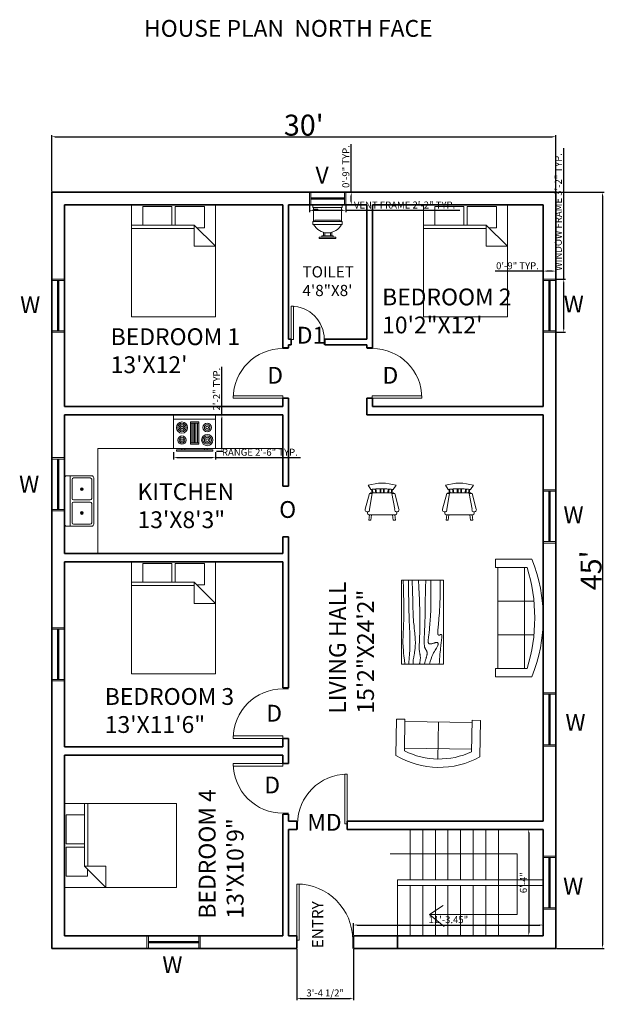
# Model space of a CAD drawing. Units: inches. Extents: x 1662 to 23131, y 1265 to 19127.
# Tile 1 of 26: x 2071 to 2489, y 1265 to 1968. Entities that reach past the tile are written whole.
import ezdxf

# ---------------------------------------------------------------- set-up
doc = ezdxf.new("R2010")
doc.units = ezdxf.units.IN
for name, color, linetype, lineweight in [('A-ANNO-DIMS', 4, 'Continuous', 18), ('A-ANNO-IDEN', 7, 'Continuous', 18), ('A-ANNO-TITL', 7, 'Continuous', 35), ('A-AREA-IDEN', 7, 'Continuous', 18), ('A-DOOR', 3, 'Continuous', 18), ('A-EQPM', 8, 'Continuous', 18), ('A-FLOR-CASE', 8, 'Continuous', 18), ('A-FLOR-FIXT', 9, 'Continuous', 18), ('A-FLOR-STRS', 7, 'Continuous', 18), ('A-FURN', 8, 'Continuous', 18), ('A-GLAZ', 4, 'Continuous', 18), ('A-WALL', 7, 'Continuous', 35)]:
    doc.layers.add(name, color=color, linetype=linetype, lineweight=lineweight)
doc.styles.get("Standard").update_dxf_attribs({"font": 'arial.ttf'})
doc.dimstyles.new('ISO-25', dxfattribs={"dimtxt": 5, "dimasz": 2.5, "dimexe": 1.25, "dimexo": 0.625, "dimtad": 1, "dimlunit": 3, "dimtxsty": 'Standard', "dimcen": 2.5, "dimadec": 0, "dimazin": 0, "dimtfac": 1, "dimtmove": 0, "dimatfit": 3, "dimfxl": 1, "dimarcsym": 0})

# ---------------------------------------------------------------- blocks, each defined once
blk = doc.blocks.new('*D1')
at = {"layer": 'A-ANNO-DIMS', "color": 0, "lineweight": -2, "transparency": 16777216}
for p, q in [((2094.29, 1845.35), (2094.29, 1885.6)), ((2454.29, 1845.35), (2454.29, 1885.6)), ((2096.79, 1884.35), (2451.79, 1884.35))]:
    blk.add_line(p, q, dxfattribs=at)
at = {"layer": 'A-ANNO-DIMS', "color": 0, "transparency": 16777216}
for points in [[(2096.79, 1884.76), (2096.79, 1883.93), (2094.29, 1884.35)], [(2451.79, 1884.76), (2451.79, 1883.93), (2454.29, 1884.35)]]:
    blk.add_solid(points, dxfattribs=at)
at = {"layer": 'Defpoints', "color": 0, "transparency": 16777216}
for p in [(2454.29, 1884.35), (2094.29, 1844.72), (2454.29, 1844.72)]:
    blk.add_point(p, dxfattribs=at)
at = {"layer": 'A-ANNO-DIMS', "color": 0, "transparency": 16777216, "insert": (2274.29, 1892.63), "char_height": 5, "attachment_point": 5}
blk.add_mtext("{\\H3x;30'}", dxfattribs=at)
blk = doc.blocks.new('*D2')
at = {"layer": 'A-ANNO-DIMS', "color": 0, "lineweight": -2, "transparency": 16777216}
for p, q in [((2454.92, 1844.72), (2488.97, 1844.72)), ((2487.72, 1842.22), (2487.72, 1307.22)), ((2454.92, 1304.72), (2488.97, 1304.72))]:
    blk.add_line(p, q, dxfattribs=at)
at = {"layer": 'A-ANNO-DIMS', "color": 0, "transparency": 16777216}
for points in [[(2487.3, 1842.22), (2488.13, 1842.22), (2487.72, 1844.72)], [(2487.3, 1307.22), (2488.13, 1307.22), (2487.72, 1304.72)]]:
    blk.add_solid(points, dxfattribs=at)
at = {"layer": 'Defpoints', "color": 0, "transparency": 16777216}
for p in [(2454.29, 1844.72), (2454.29, 1304.72), (2487.72, 1304.72)]:
    blk.add_point(p, dxfattribs=at)
at = {"layer": 'A-ANNO-DIMS', "color": 0, "transparency": 16777216, "insert": (2479.46, 1574.72), "char_height": 5, "attachment_point": 5, "rotation": 90}
blk.add_mtext("{\\H3x;45'}", dxfattribs=at)
blk = doc.blocks.new('*U4')
for p, q in [((0, 0), (0, -100)), ((-900, 0), (-900, -100))]:
    blk.add_line(p, q)
blk.add_lwpolyline([(0, 0), (0, 900), (-43.75, 900), (-43.75, 0)], close=True)
blk.add_arc((0, 0), 900, 90, 180)
blk = doc.blocks.new('*U5')
for p, q in [((-900, 0), (-900, 100)), ((0, 0), (0, 100))]:
    blk.add_line(p, q)
blk.add_lwpolyline([(0, 0), (0, -900), (-43.75, -900), (-43.75, 0)], close=True)
blk.add_arc((0, 0), 900, 180, 270)
blk = doc.blocks.new('*U6')
for p, q in [((0, 0), (0, 100)), ((900, 0), (900, 100))]:
    blk.add_line(p, q)
blk.add_lwpolyline([(0, 0), (0, -900), (43.75, -900), (43.75, 0)], close=True)
blk.add_arc((0, 0), 900, 270, 0)
blk = doc.blocks.new('*U7')
for p, q in [((0, 0), (0, -100)), ((-900, 0), (-900, -100))]:
    blk.add_line(p, q)
blk.add_lwpolyline([(0, 0), (0, 900), (-43.75, 900), (-43.75, 0)], close=True)
blk.add_arc((0, 0), 900, 90, 180)
blk = doc.blocks.new('*U8')
for p, q in [((0, 0), (0, -100)), ((600, 0), (600, -100))]:
    blk.add_line(p, q)
blk.add_lwpolyline([(0, 0), (0, 600), (43.75, 600), (43.75, 0)], close=True)
blk.add_arc((0, 0), 600, 0, 90)
blk = doc.blocks.new('*U10')
for p, q in [((0, 0), (0, -6)), ((40, 0), (40, -6))]:
    blk.add_line(p, q)
blk.add_lwpolyline([(0, 0), (0, 40), (1.75, 40), (1.75, 0)], close=True)
blk.add_arc((0, 0), 40, 0, 90)
blk = doc.blocks.new('Chair - Rocking')
for p, q in [((-8, -4.5), (-10, -1.5)), ((-8.23428, -6.99939), (-8.3093, -7.47958)), ((-8.23041, -7), (8.23915, -7)), ((-7.5, -4.5), (-7, -7)), ((-6.5, -7), (-7.02225, -4.43)), ((-4.5, -7), (-4.96674, -4.19951)), ((-4, -7), (-4.40532, -4.16272)), ((-1.5, -4.05012), (-1.5, -7)), ((-1, -7), (-1, -4.05012)), ((1, -7), (1, -4.04655)), ((1.5, -4.05012), (1.5, -7)), ((4, -7), (4.40187, -4.18694)), ((4.5, -7), (4.96761, -4.19437)), ((6.5, -7), (7, -4.4057)), ((7.5, -4.5), (7, -7)), ((8, -4.5), (10, -1.5)), ((8.31071, -7.48854), (8.23449, -7.00073)), ((-9, -7.5), (-12, -18.49999)), ((-7, -7.5), (-9, -7.5)), ((-9, -18.49999), (-7, -7.5)), ((7, -7.5), (9, -7.5)), ((9, -18.49999), (7, -7.5)), ((9, -7.5), (12, -18.49999)), ((-10.36644, -20.64523), (-10.5, -21.49999)), ((10.5, -21.49999), (10.3575, -20.58798)), ((-9, -22.49999), (-9.5, -26.49999)), ((0, -22.49999), (-9.5, -22.49999)), ((-9.5, -26.49999), (-8, -26.49999)), ((-8, -26.49999), (-7.5, -22.49999)), ((0, -22.49999), (9.5, -22.49999)), ((8, -26.49999), (7.5, -22.49999)), ((9.5, -26.49999), (8, -26.49999)), ((9, -22.49999), (9.5, -26.49999))]:
    blk.add_line(p, q)
for centre, radius, start, end in [((0, -34.08333), 34.08333, 72.93847, 107.0615), ((0, -68.25004), 64.25, 93.92211, 97.15267), ((0, -68.25004), 64.25, 82.84733, 93.92211), ((-10.5, -18.99999), 1.58114, 161.5651, 18.43495), ((10.5, -18.99999), 1.58114, 161.5651, 18.43495), ((-9.5, -21.49999), 1, 180, 270), ((9.5, -21.49999), 1, 270, 0)]:
    blk.add_arc(centre, radius, start, end)
blk = doc.blocks.new('Table - Rectangular Woodgrain 60 x 30 in.')
for p, q in [((0, 0), (0, -30)), ((60, 0), (0, 0)), ((60, -30), (60, 0)), ((0, -30), (60, -30))]:
    blk.add_line(p, q)
for points in [[(0, -2.4), (4.8155, -2.418), (9.0302, -2.4688), (12.709, -2.5477), (15.9167, -2.65), (18.7181, -2.7711), (21.1781, -2.9063), (23.3616, -3.0508), (25.3333, -3.2), (27.1477, -3.3495), (28.8172, -3.4958), (30.3437, -3.636), (31.7291, -3.7667), (32.9756, -3.8849), (34.0849, -3.9875), (35.059, -4.0714), (35.9, -4.1334), (36.6114, -4.1711), (37.2041, -4.1854), (37.6906, -4.1779), (38.0833, -4.15), (38.3948, -4.1034), (38.6375, -4.0396), (38.8239, -3.9602), (38.9666, -3.8667), (39.0764, -3.7608), (39.1573, -3.6448), (39.2116, -3.521), (39.2416, -3.3917), (39.2498, -3.2593), (39.2385, -3.1261), (39.21, -2.9944), (39.1666, -2.8667), (39.111, -2.7447), (39.0468, -2.6281), (38.978, -2.5163), (38.9083, -2.4083), (38.8418, -2.3035), (38.7823, -2.201), (38.7337, -2.1001), (38.7, -2), (38.6844, -1.9003), (38.6875, -1.8021), (38.7094, -1.707), (38.75, -1.6167), (38.8094, -1.5326), (38.8875, -1.4563), (38.9844, -1.3893), (39.1, -1.3333), (39.2351, -1.2896), (39.3937, -1.2583), (39.5804, -1.2396), (39.8, -1.2333), (40.057, -1.2396), (40.3562, -1.2583), (40.7023, -1.2896), (41.1, -1.3333), (41.5547, -1.3895), (42.0755, -1.4573), (42.6721, -1.5361), (43.3542, -1.625), (44.1316, -1.7233), (45.014, -1.8302), (46.0114, -1.9449), (47.1333, -2.0667), (48.3862, -2.1947), (49.7625, -2.3281), (51.2513, -2.4663), (52.8416, -2.6083), (54.5226, -2.7535), (56.2833, -2.9011), (58.1127, -3.0501), (60, -3.2)], [(0, -9.2), (6.5759, -9.0858), (11.9385, -9.0365), (16.2527, -9.0418), (19.6833, -9.0917), (22.3952, -9.1759), (24.5531, -9.2844), (26.322, -9.4069), (27.8666, -9.5333), (29.3241, -9.6553), (30.7203, -9.7719), (32.0532, -9.8837), (33.3208, -9.9917), (34.5213, -10.0965), (35.6526, -10.199), (36.7128, -10.2999), (37.7, -10.4), (38.6129, -10.4996), (39.4531, -10.5969), (40.223, -10.6895), (40.925, -10.775), (41.5613, -10.8512), (42.1344, -10.9156), (42.6465, -10.966), (43.1, -11), (43.4976, -11.0158), (43.8437, -11.0136), (44.143, -10.9942), (44.4, -10.9583), (44.6195, -10.9069), (44.8062, -10.8406), (44.9648, -10.7603), (45.1, -10.6667), (45.2155, -10.5598), (45.3114, -10.4365), (45.3871, -10.2929), (45.4416, -10.125), (45.4743, -9.929), (45.4844, -9.7011), (45.4709, -9.4371), (45.4333, -9.1333), (45.3716, -8.7883), (45.2896, -8.4104), (45.1919, -8.0107), (45.0833, -7.6), (44.9685, -7.1893), (44.8521, -6.7896), (44.7388, -6.4117), (44.6333, -6.0667), (44.54, -5.7628), (44.4614, -5.4979), (44.4001, -5.2675), (44.3583, -5.0667), (44.3384, -4.8909), (44.3427, -4.7354), (44.3736, -4.5956), (44.4333, -4.4667), (44.5236, -4.3453), (44.6427, -4.2333), (44.7884, -4.1339), (44.9583, -4.05), (45.1501, -3.9849), (45.3614, -3.9417), (45.59, -3.9234), (45.8333, -3.9333), (46.0915, -3.9749), (46.3734, -4.0531), (46.6906, -4.1736), (47.0542, -4.3417), (47.4756, -4.5629), (47.9661, -4.8427), (48.5372, -5.1866), (49.2, -5.6), (49.9676, -6.0844), (50.8594, -6.625), (51.8965, -7.2031), (53.1, -7.8), (54.491, -8.3969), (56.0906, -8.975), (57.9199, -9.5156), (60, -10)], [(0, -12.8), (5.1847, -12.9322), (9.6213, -13.0323), (13.3963, -13.1059), (16.5958, -13.1583), (19.3063, -13.1952), (21.614, -13.2219), (23.6054, -13.2439), (25.3666, -13.2667), (26.9728, -13.2947), (28.4531, -13.3281), (29.8256, -13.3663), (31.1083, -13.4083), (32.3191, -13.4535), (33.476, -13.501), (34.597, -13.5501), (35.7, -13.6), (36.7984, -13.6497), (37.8875, -13.6979), (38.9578, -13.743), (40, -13.7833), (41.0047, -13.8174), (41.9625, -13.8438), (42.864, -13.8607), (43.7, -13.8667), (44.4631, -13.8604), (45.1552, -13.8417), (45.7801, -13.8104), (46.3416, -13.7667), (46.8439, -13.7104), (47.2906, -13.6417), (47.6858, -13.5604), (48.0333, -13.4667), (48.3375, -13.3608), (48.6042, -13.2448), (48.8396, -13.121), (49.05, -12.9917), (49.2417, -12.8593), (49.4208, -12.7261), (49.5937, -12.5944), (49.7667, -12.4667), (49.9452, -12.3451), (50.1323, -12.2313), (50.3303, -12.1268), (50.5416, -12.0333), (50.7686, -11.9524), (51.0135, -11.8854), (51.2788, -11.8341), (51.5666, -11.8), (51.8785, -11.7843), (52.2116, -11.7865), (52.562, -11.8059), (52.926, -11.8417), (53.2998, -11.8931), (53.6795, -11.9594), (54.0614, -12.0397), (54.4416, -12.1333), (54.8223, -12.2401), (55.2293, -12.3625), (55.6942, -12.5037), (56.2489, -12.6667), (56.9251, -12.8547), (57.7545, -13.0708), (58.7689, -13.3182), (60, -13.6)], [(0, -18), (5.124, -17.7273), (9.6609, -17.5057), (13.6705, -17.3303), (17.2125, -17.1958), (20.3467, -17.0973), (23.1328, -17.0297), (25.6307, -16.9878), (27.9, -16.9667), (29.9928, -16.9617), (31.9302, -16.9703), (33.7254, -16.9907), (35.3917, -17.0208), (36.9423, -17.0588), (38.3906, -17.1026), (39.7499, -17.1503), (41.0333, -17.2), (42.2519, -17.2496), (43.4073, -17.2969), (44.4986, -17.3395), (45.525, -17.375), (46.4858, -17.4012), (47.3802, -17.4156), (48.2074, -17.416), (48.9667, -17.4), (49.6583, -17.3662), (50.2872, -17.3167), (50.8595, -17.2547), (51.3812, -17.1833), (51.8584, -17.1057), (52.2971, -17.025), (52.7034, -16.9443), (53.0833, -16.8667), (53.443, -16.7951), (53.789, -16.7313), (54.128, -16.6768), (54.4666, -16.6334), (54.8115, -16.6024), (55.1693, -16.5854), (55.5465, -16.5841), (55.95, -16.6), (56.3828, -16.6337), (56.8346, -16.6823), (57.2915, -16.7418), (57.7396, -16.8084), (58.165, -16.878), (58.5539, -16.9469), (58.8924, -17.0111), (59.1666, -17.0667), (59.3679, -17.1107), (59.5078, -17.1438), (59.6032, -17.1675), (59.6708, -17.1833), (59.7275, -17.193), (59.7901, -17.1979), (59.8753, -17.1998), (60, -17.2)], [(0, -22.4), (8.0098, -22.2501), (14.4094, -22.1011), (19.4168, -21.9535), (23.25, -21.8083), (26.1269, -21.6663), (28.2656, -21.5281), (29.884, -21.3947), (31.2, -21.2667), (32.3967, -21.1448), (33.5172, -21.0292), (34.5697, -20.9198), (35.5625, -20.8167), (36.5037, -20.7198), (37.4015, -20.6292), (38.2642, -20.5448), (39.1, -20.4667), (39.9164, -20.3951), (40.7187, -20.3313), (41.5117, -20.2768), (42.3, -20.2333), (43.0883, -20.2024), (43.8812, -20.1854), (44.6836, -20.1841), (45.5, -20.2), (46.3328, -20.234), (47.1747, -20.2844), (48.0163, -20.3488), (48.8479, -20.425), (49.66, -20.5106), (50.4429, -20.6031), (51.1872, -20.7004), (51.8833, -20.8), (52.5246, -20.8999), (53.1166, -20.9995), (53.6681, -21.0983), (54.1875, -21.1958), (54.6834, -21.2919), (55.1646, -21.3859), (55.6394, -21.4777), (56.1167, -21.5667), (56.6028, -21.6515), (57.0961, -21.7266), (57.5929, -21.7852), (58.0896, -21.8208), (58.5823, -21.8268), (59.0674, -21.7964), (59.5412, -21.723), (60, -21.6)], [(0, -25.2), (8.6355, -25.0504), (15.7026, -24.9031), (21.4049, -24.7606), (25.9458, -24.625), (29.529, -24.4988), (32.3578, -24.3844), (34.6359, -24.284), (36.5667, -24.2), (38.3213, -24.1341), (39.9417, -24.0854), (41.437, -24.0523), (42.8167, -24.0333), (44.0901, -24.0268), (45.2667, -24.0313), (46.3557, -24.0451), (47.3667, -24.0667), (48.309, -24.0947), (49.1928, -24.1287), (50.0284, -24.168), (50.826, -24.2125), (51.5959, -24.2617), (52.3483, -24.3151), (53.0935, -24.3725), (53.8417, -24.4334), (54.6009, -24.497), (55.3699, -24.561), (56.1454, -24.6226), (56.9239, -24.6792), (57.7021, -24.7279), (58.4764, -24.7662), (59.2435, -24.7911), (60, -24.8)], [(0, -28.8), (5.6867, -28.6681), (10.45, -28.5698), (14.407, -28.5012), (17.675, -28.4584), (20.3711, -28.4374), (22.6125, -28.4344), (24.5164, -28.4455), (26.2, -28.4667), (27.762, -28.4947), (29.2276, -28.5281), (30.6033, -28.5663), (31.8958, -28.6084), (33.1118, -28.6535), (34.2578, -28.7011), (35.3405, -28.7501), (36.3666, -28.8), (37.3443, -28.8497), (38.288, -28.8974), (39.2137, -28.9412), (40.1375, -28.9792), (41.0753, -29.0093), (42.0432, -29.0297), (43.0572, -29.0384), (44.1333, -29.0333), (45.2936, -29.0114), (46.5843, -28.9641), (48.0579, -28.8816), (49.7666, -28.7542), (51.7629, -28.5721), (54.0989, -28.3255), (56.8272, -28.0048), (60, -27.6)]]:
    blk.add_lwpolyline(points)
blk = doc.blocks.new('Sink-double - 36 in top')
for p, q in [((-18, -4), (18, -4)), ((-0.75, -18.5), (-0.75, -6.5)), ((0.75, -6.5), (0.75, -18.5))]:
    blk.add_line(p, q)
for points in [[(-16.5, 0), (16.5, 0)], [(-18, -19.5), (-18, -1.5)], [(-16.5, -18.5), (-16.5, -6.5)], [(-15.5, -5.5), (-1.75, -5.5)], [(1.75, -5.5), (15.5, -5.5)], [(16.5, -6.5), (16.5, -18.5)], [(18, -1.5), (18, -19.5)], [(16.5, -21), (-16.5, -21)], [(-1.75, -19.5), (-15.5, -19.5)], [(15.5, -19.5), (1.75, -19.5)]]:
    blk.add_lwpolyline(points)
for centre, radius in [((-8.5, -12.5), 1), ((-8.5, -12.5), 0.5), ((8.5, -12.5), 1), ((8.5, -12.5), 0.5)]:
    blk.add_circle(centre, radius)
for centre, radius, start, end in [((-16.5, -1.5), 1.5, 90, 180), ((16.5, -1.5), 1.5, 0, 90), ((-15.5, -6.5), 1, 90, 180), ((-1.75, -6.5), 1, 0, 90), ((1.75, -6.5), 1, 90, 180), ((15.5, -6.5), 1, 0, 90), ((-16.5, -19.5), 1.5, 180, 270), ((-15.5, -18.5), 1, 180, 270), ((-1.75, -18.5), 1, 270, 0), ((1.75, -18.5), 1, 180, 270), ((15.5, -18.5), 1, 270, 0), ((16.5, -19.5), 1.5, 270, 0)]:
    blk.add_arc(centre, radius, start, end)
blk = doc.blocks.new('Range-Oven - 30 in top')
for p, q in [((0, -3), (30, -3)), ((12, -6), (18, -6)), ((13, -20), (13, -6)), ((14, -6), (14, -20)), ((15, -20), (15, -6)), ((16, -6), (16, -20)), ((17, -20), (17, -6)), ((18, -20), (12, -20)), ((6, -24), (6, -25)), ((8, -25), (8, -24)), ((22, -25), (22, -24)), ((24, -24), (24, -25))]:
    blk.add_line(p, q)
for points in [[(0, -24), (0, 0), (30, 0), (30, -24)], [(12, -21), (12, -5), (18, -5), (18, -21)], [(2, -26), (2, -25), (28, -25), (28, -26)]]:
    blk.add_lwpolyline(points, close=True)
for centre, radius in [((6, -9), 4), ((6, -9), 3), ((6, -9), 2), ((24, -9), 3), ((24, -9), 2), ((6, -9), 1), ((24, -18), 4), ((24, -9), 1), ((6, -18), 3), ((6, -18), 2), ((6, -18), 1), ((24, -18), 3), ((24, -18), 2), ((24, -18), 1)]:
    blk.add_circle(centre, radius)
blk = doc.blocks.new('Bed - Queen')
for p, q in [((0, -80.00003), (0, 0)), ((0, 0), (59.99999, 0)), ((59.99999, 0), (59.99999, -80.00003)), ((7.99999, -1.2), (28.79998, -1.2)), ((7.99999, -14.4), (7.99999, -1.2)), ((28.79998, -1.2), (28.79998, -14.4)), ((31.19999, -1.2), (51.99999, -1.2)), ((31.19999, -14.4), (31.19999, -1.2)), ((51.99999, -1.2), (51.99999, -16.4)), ((0, -14.4), (44.8, -14.4)), ((44.8, -16.8), (0, -16.8)), ((59.99999, -29.6), (44.8, -14.4)), ((44.8, -14.4), (44.8, -29.6)), ((51.99999, -16.4), (46.79936, -16.4)), ((44.8, -29.6), (59.99999, -29.6)), ((59.99999, -80.00003), (0, -80.00003))]:
    blk.add_line(p, q)
blk = doc.blocks.new('*U13')
for p, q in [((-254, 558.8), (-254, 304.8)), ((254, 304.8), (254, 558.8)), ((-254, 533.4), (-177.8, 533.4)), ((-177.8, 508), (-254, 508)), ((-177.8, 533.4), (-177.8, 508)), ((266.7, 304.8), (-266.7, 304.8)), ((-266.7, 254), (-266.7, 304.8)), ((266.7, 254), (-266.7, 254)), ((228.6, 330.2), (-228.6, 330.2)), ((-228.6, 330.2), (-228.6, 304.8)), ((228.6, 304.8), (228.6, 330.2)), ((266.7, 304.8), (266.7, 254)), ((101.6, 50.8), (-101.6, 50.8)), ((-101.6, 50.8), (-101.6, 25.4)), ((-76.2, 111.9251), (-76.2, 50.8)), ((-50.8, 50.8), (-50.8, 105.81132)), ((50.8, 105.81132), (50.8, 50.8)), ((76.2, 50.8), (76.2, 111.9251)), ((101.6, 25.4), (101.6, 50.8))]:
    blk.add_line(p, q)
for points in [[(266.7, 558.8), (266.7, 609.6), (-266.7, 609.6), (-266.7, 558.8)], [(152.4, 0), (152.4, 25.4), (-152.4, 25.4), (-152.4, 0)]]:
    blk.add_lwpolyline(points, close=True)
blk.add_arc((0, 389.46582), 287.86658, 208.0725, 331.9275)
blk = doc.blocks.new('Sofa - Roundback 7 ft.')
for p, q in [((-12.00002, -32.4421), (-12.00003, -6.5971)), ((11.99997, -32.4421), (11.99998, -6.5971)), ((-36.000027, -34), (-36.000027, -11.4696)), ((-35.999844, -13.3819), (35.9998, -13.3819)), ((35.99998, -34), (35.99998, -11.4696)), ((-36.000027, -32.4421), (35.99998, -32.4421))]:
    blk.add_line(p, q)
for points in [[(-36.000027, -34), (-42.000027, -34), (-42.000027, -8)], [(41.99998, -8), (41.99998, -34), (35.99998, -34)]]:
    blk.add_lwpolyline(points)
for centre, radius, start, end in [((0, -114.25), 114.25, 68.43141, 111.5686), ((-0.00001, -127.1968), 121.1968, 72.72033, 107.2797)]:
    blk.add_arc(centre, radius, start, end)
blk = doc.blocks.new('Sofa - Roundback Loveseat 5 ft.')
for p, q in [((0, -32.44198), (0, -5.99998)), ((-24, -33.99998), (-24, -11.46958)), ((-23.9998, -13.38178), (23.99986, -13.38178)), ((24.00004, -33.99998), (24.00004, -11.46958)), ((-24, -32.44198), (24.00004, -32.44198))]:
    blk.add_line(p, q)
for points in [[(-24, -33.99998), (-30, -33.99998), (-30, -7.99998)], [(30.00004, -7.99998), (30.00004, -33.99998), (24.00004, -33.99998)]]:
    blk.add_lwpolyline(points)
for centre, radius, start, end in [((0, -60.24998), 60.24998, 60.13715, 119.8628), ((0, -61.38438), 55.38444, 64.32083, 115.6792)]:
    blk.add_arc(centre, radius, start, end)
blk = doc.blocks.new('*D23')
at = {"layer": 'A-ANNO-DIMS', "color": 0, "lineweight": -2, "transparency": 16777216}
for p, q in [((2309.85, 1314.35), (2309.85, 1322.7)), ((2445.29, 1314.35), (2445.29, 1322.7)), ((2312.35, 1321.45), (2442.79, 1321.45))]:
    blk.add_line(p, q, dxfattribs=at)
at = {"layer": 'A-ANNO-DIMS', "color": 0, "transparency": 16777216}
for points in [[(2312.35, 1321.87), (2312.35, 1321.04), (2309.85, 1321.45)], [(2442.79, 1321.87), (2442.79, 1321.04), (2445.29, 1321.45)]]:
    blk.add_solid(points, dxfattribs=at)
at = {"layer": 'Defpoints', "color": 0, "transparency": 16777216}
for p in [(2445.29, 1321.45), (2309.85, 1313.72), (2445.29, 1313.72)]:
    blk.add_point(p, dxfattribs=at)
at = {"layer": 'A-ANNO-DIMS', "color": 0, "transparency": 16777216, "insert": (2377.57, 1324.63), "char_height": 5, "attachment_point": 5}
blk.add_mtext('11\'-3.45"', dxfattribs=at)
blk = doc.blocks.new('*D24')
at = {"layer": 'A-ANNO-DIMS', "color": 0, "lineweight": -2, "transparency": 16777216}
for p, q in [((2444.67, 1389.72), (2433.72, 1389.72)), ((2434.97, 1387.22), (2434.97, 1316.22)), ((2444.67, 1313.72), (2433.72, 1313.72))]:
    blk.add_line(p, q, dxfattribs=at)
at = {"layer": 'A-ANNO-DIMS', "color": 0, "transparency": 16777216}
for points in [[(2434.56, 1387.22), (2435.39, 1387.22), (2434.97, 1389.72)], [(2434.56, 1316.22), (2435.39, 1316.22), (2434.97, 1313.72)]]:
    blk.add_solid(points, dxfattribs=at)
at = {"layer": 'Defpoints', "color": 0, "transparency": 16777216}
for p in [(2445.29, 1389.72), (2434.97, 1313.72), (2445.29, 1313.72)]:
    blk.add_point(p, dxfattribs=at)
at = {"layer": 'A-ANNO-DIMS', "color": 0, "transparency": 16777216, "insert": (2431.8, 1351.72), "char_height": 5, "attachment_point": 5, "rotation": 90}
blk.add_mtext('6\'-4"', dxfattribs=at)
blk = doc.blocks.new('WIN-36-J9X1')
for p, q in [((0, 9), (0, 0)), ((1, 9), (1, 0)), ((37, 9), (37, 0)), ((38, 9), (38, 0)), ((1, 5), (37, 5)), ((1, 4.5), (37, 4.5)), ((1, 4), (37, 4))]:
    blk.add_line(p, q)
blk = doc.blocks.new('VENT-24-J9X1')
for p, q in [((0, 9), (0, 0)), ((1, 9), (1, 0)), ((25, 9), (25, 0)), ((26, 9), (26, 0)), ((1, 5), (25, 5)), ((1, 4.5), (25, 4.5)), ((1, 4), (25, 4))]:
    blk.add_line(p, q)
blk = doc.blocks.new('*D159')
at = {"layer": 'A-ANNO-DIMS', "color": 0, "lineweight": -2, "transparency": 16777216}
for p, q in [((2459.99, 1782.72), (2459.99, 1876.13)), ((2454.92, 1782.72), (2461.24, 1782.72)), ((2459.99, 1747.22), (2459.99, 1780.22)), ((2454.92, 1744.72), (2461.24, 1744.72))]:
    blk.add_line(p, q, dxfattribs=at)
at = {"layer": 'A-ANNO-DIMS', "color": 0, "transparency": 16777216}
for points in [[(2459.58, 1780.22), (2460.41, 1780.22), (2459.99, 1782.72)], [(2459.58, 1747.22), (2460.41, 1747.22), (2459.99, 1744.72)]]:
    blk.add_solid(points, dxfattribs=at)
at = {"layer": 'Defpoints', "color": 0, "transparency": 16777216}
for p in [(2454.29, 1782.72), (2459.99, 1782.72), (2454.29, 1744.72)]:
    blk.add_point(p, dxfattribs=at)
at = {"layer": 'A-ANNO-DIMS', "color": 0, "transparency": 16777216, "insert": (2456.78, 1830.67), "char_height": 5, "attachment_point": 5, "rotation": 90}
blk.add_mtext('WINDOW FRAME 3\'-2" TYP.', dxfattribs=at)
blk = doc.blocks.new('*D160')
at = {"layer": 'A-ANNO-DIMS', "color": 0, "lineweight": -2, "transparency": 16777216}
for p, q in [((2445.29, 1788.42), (2411.07, 1788.42)), ((2445.29, 1783.35), (2445.29, 1789.67)), ((2451.79, 1788.42), (2447.79, 1788.42)), ((2454.29, 1783.35), (2454.29, 1789.67))]:
    blk.add_line(p, q, dxfattribs=at)
at = {"layer": 'A-ANNO-DIMS', "color": 0, "transparency": 16777216}
for points in [[(2447.79, 1788.84), (2447.79, 1788), (2445.29, 1788.42)], [(2451.79, 1788.84), (2451.79, 1788), (2454.29, 1788.42)]]:
    blk.add_solid(points, dxfattribs=at)
at = {"layer": 'Defpoints', "color": 0, "transparency": 16777216}
for p in [(2445.29, 1788.42), (2445.29, 1782.72), (2454.29, 1782.72)]:
    blk.add_point(p, dxfattribs=at)
at = {"layer": 'A-ANNO-DIMS', "color": 0, "transparency": 16777216, "insert": (2426.93, 1791.6), "char_height": 5, "attachment_point": 5}
blk.add_mtext('0\'-9" TYP.', dxfattribs=at)
blk = doc.blocks.new('*D171')
at = {"layer": 'A-ANNO-DIMS', "color": 0, "lineweight": -2, "transparency": 16777216}
for p, q in [((2278.29, 1835.1), (2278.29, 1830.57)), ((2280.79, 1831.82), (2301.79, 1831.82)), ((2304.29, 1835.1), (2304.29, 1830.57)), ((2304.29, 1831.82), (2385.74, 1831.82))]:
    blk.add_line(p, q, dxfattribs=at)
at = {"layer": 'A-ANNO-DIMS', "color": 0, "transparency": 16777216}
for points in [[(2280.79, 1832.24), (2280.79, 1831.4), (2278.29, 1831.82)], [(2301.79, 1832.24), (2301.79, 1831.4), (2304.29, 1831.82)]]:
    blk.add_solid(points, dxfattribs=at)
at = {"layer": 'Defpoints', "color": 0, "transparency": 16777216}
for p in [(2278.29, 1835.72), (2304.29, 1835.72), (2304.29, 1831.82)]:
    blk.add_point(p, dxfattribs=at)
at = {"layer": 'A-ANNO-DIMS', "color": 0, "transparency": 16777216, "insert": (2346.27, 1834.96), "char_height": 5, "attachment_point": 5}
blk.add_mtext('VENT FRAME 2\'-2" TYP.', dxfattribs=at)
blk = doc.blocks.new('*D172')
at = {"layer": 'A-ANNO-DIMS', "color": 0, "lineweight": -2, "transparency": 16777216}
for p, q in [((2308.19, 1844.72), (2308.19, 1878.95)), ((2304.92, 1844.72), (2309.44, 1844.72)), ((2308.19, 1838.22), (2308.19, 1842.22)), ((2304.92, 1835.72), (2309.44, 1835.72))]:
    blk.add_line(p, q, dxfattribs=at)
at = {"layer": 'A-ANNO-DIMS', "color": 0, "transparency": 16777216}
for points in [[(2307.78, 1842.22), (2308.61, 1842.22), (2308.19, 1844.72)], [(2307.78, 1838.22), (2308.61, 1838.22), (2308.19, 1835.72)]]:
    blk.add_solid(points, dxfattribs=at)
at = {"layer": 'Defpoints', "color": 0, "transparency": 16777216}
for p in [(2304.29, 1844.72), (2308.19, 1844.72), (2304.29, 1835.72)]:
    blk.add_point(p, dxfattribs=at)
at = {"layer": 'A-ANNO-DIMS', "color": 0, "transparency": 16777216, "insert": (2305.02, 1863.08), "char_height": 5, "attachment_point": 5, "rotation": 90}
blk.add_mtext('0\'-9" TYP.', dxfattribs=at)
blk = doc.blocks.new('*D183')
at = {"layer": 'A-ANNO-DIMS', "color": 0, "lineweight": -2, "transparency": 16777216}
for p, q in [((2181.29, 1659.1), (2181.29, 1653.97)), ((2183.79, 1655.22), (2208.79, 1655.22)), ((2211.29, 1659.1), (2211.29, 1653.97)), ((2211.29, 1655.22), (2272.04, 1655.22))]:
    blk.add_line(p, q, dxfattribs=at)
at = {"layer": 'A-ANNO-DIMS', "color": 0, "transparency": 16777216}
for points in [[(2183.79, 1655.64), (2183.79, 1654.8), (2181.29, 1655.22)], [(2208.79, 1655.64), (2208.79, 1654.8), (2211.29, 1655.22)]]:
    blk.add_solid(points, dxfattribs=at)
at = {"layer": 'Defpoints', "color": 0, "transparency": 16777216}
for p in [(2181.29, 1659.72), (2211.29, 1659.72), (2211.29, 1655.22)]:
    blk.add_point(p, dxfattribs=at)
at = {"layer": 'A-ANNO-DIMS', "color": 0, "transparency": 16777216, "insert": (2242.92, 1658.43), "char_height": 5, "attachment_point": 5}
blk.add_mtext('RANGE 2\'-6" TYP.', dxfattribs=at)
blk = doc.blocks.new('*D184')
at = {"layer": 'A-ANNO-DIMS', "color": 0, "lineweight": -2, "transparency": 16777216}
for p, q in [((2215.79, 1685.72), (2215.79, 1720.03)), ((2211.92, 1685.72), (2217.04, 1685.72)), ((2215.79, 1662.22), (2215.79, 1683.22)), ((2211.92, 1659.72), (2217.04, 1659.72))]:
    blk.add_line(p, q, dxfattribs=at)
at = {"layer": 'A-ANNO-DIMS', "color": 0, "transparency": 16777216}
for points in [[(2215.38, 1683.22), (2216.21, 1683.22), (2215.79, 1685.72)], [(2215.38, 1662.22), (2216.21, 1662.22), (2215.79, 1659.72)]]:
    blk.add_solid(points, dxfattribs=at)
at = {"layer": 'Defpoints', "color": 0, "transparency": 16777216}
for p in [(2211.29, 1685.72), (2215.79, 1685.72), (2211.29, 1659.72)]:
    blk.add_point(p, dxfattribs=at)
at = {"layer": 'A-ANNO-DIMS', "color": 0, "transparency": 16777216, "insert": (2212.66, 1704.13), "char_height": 5, "attachment_point": 5, "rotation": 90}
blk.add_mtext('2\'-2" TYP.', dxfattribs=at)
blk = doc.blocks.new('*D207')
at = {"layer": 'A-ANNO-DIMS', "color": 0, "lineweight": -2, "transparency": 16777216}
for p, q in [((2269.29, 1304.1), (2269.29, 1267.82)), ((2309.85, 1304.1), (2309.85, 1267.82)), ((2271.79, 1269.07), (2307.35, 1269.07))]:
    blk.add_line(p, q, dxfattribs=at)
at = {"layer": 'A-ANNO-DIMS', "color": 0, "transparency": 16777216}
for points in [[(2271.79, 1269.49), (2271.79, 1268.65), (2269.29, 1269.07)], [(2307.35, 1269.49), (2307.35, 1268.65), (2309.85, 1269.07)]]:
    blk.add_solid(points, dxfattribs=at)
at = {"layer": 'Defpoints', "color": 0, "transparency": 16777216}
for p in [(2269.29, 1304.72), (2309.85, 1304.72), (2309.85, 1269.07)]:
    blk.add_point(p, dxfattribs=at)
at = {"layer": 'A-ANNO-DIMS', "color": 0, "transparency": 16777216, "insert": (2289.57, 1272.28), "char_height": 5, "attachment_point": 5}
blk.add_mtext('3\'-4 1/2"', dxfattribs=at)

msp = doc.modelspace()

# ---------------------------------------------------------------- linework, layer by layer
at = {"layer": 'A-FLOR-CASE'}
for p, q in [((2127.295, 1586.72), (2127.295, 1661.72)), ((2127.295, 1661.72), (2259.295, 1661.72))]:
    msp.add_line(p, q, dxfattribs=at)
at = {"layer": 'A-FLOR-STRS'}
for p, q in [((2350.295, 1353.72), (2350.295, 1389.72)), ((2359.295, 1353.72), (2359.295, 1389.72)), ((2368.295, 1353.72), (2368.295, 1389.72)), ((2377.295, 1353.72), (2377.295, 1389.72)), ((2386.295, 1353.72), (2386.295, 1389.72)), ((2395.295, 1353.72), (2395.295, 1389.72)), ((2404.295, 1353.72), (2404.295, 1389.72)), ((2413.295, 1313.72), (2413.295, 1389.72)), ((2335.989, 1372.197), (2426.78, 1372.197)), ((2426.78, 1372.197), (2426.78, 1328.927)), ((2341.295, 1313.72), (2341.295, 1353.72)), ((2445.295, 1353.72), (2341.295, 1353.72)), ((2445.295, 1349.72), (2341.295, 1349.72)), ((2350.295, 1313.72), (2350.295, 1349.72)), ((2359.295, 1313.72), (2359.295, 1349.72)), ((2368.295, 1313.72), (2368.295, 1349.72)), ((2377.295, 1313.72), (2377.295, 1349.72)), ((2386.295, 1313.72), (2386.295, 1349.72)), ((2395.295, 1313.72), (2395.295, 1349.72)), ((2404.295, 1313.72), (2404.295, 1349.72)), ((2364.002, 1328.927), (2373.738, 1335.484)), ((2426.78, 1328.927), (2364.002, 1328.927)), ((2364.002, 1328.927), (2374.662, 1320.507))]:
    msp.add_line(p, q, dxfattribs=at)
at = {"layer": 'A-WALL'}
for p, q in [((2094.295, 1844.72), (2454.295, 1844.72)), ((2094.295, 1304.72), (2094.295, 1844.72)), ((2454.295, 1844.72), (2454.295, 1304.72)), ((2103.295, 1835.72), (2259.295, 1835.72)), ((2103.295, 1691.72), (2103.295, 1835.72)), ((2259.295, 1733.72), (2259.295, 1835.72)), ((2263.295, 1739.72), (2263.295, 1835.72)), ((2263.295, 1835.72), (2319.295, 1835.72)), ((2319.295, 1739.72), (2319.295, 1835.72)), ((2323.295, 1733.72), (2323.295, 1835.72)), ((2323.295, 1835.72), (2445.295, 1835.72)), ((2445.295, 1835.72), (2445.295, 1691.72)), ((2263.295, 1739.72), (2265.295, 1739.72)), ((2265.295, 1739.72), (2265.295, 1735.72)), ((2289.295, 1739.72), (2289.295, 1735.72)), ((2289.295, 1739.72), (2319.295, 1739.72)), ((2259.295, 1733.72), (2263.295, 1733.72)), ((2263.295, 1735.72), (2265.295, 1735.72)), ((2263.295, 1733.72), (2263.295, 1735.72)), ((2289.295, 1735.72), (2319.295, 1735.72)), ((2319.295, 1733.72), (2319.295, 1735.72)), ((2319.295, 1733.72), (2323.295, 1733.72)), ((2259.295, 1697.72), (2263.295, 1697.72)), ((2259.295, 1691.72), (2259.295, 1697.72)), ((2263.295, 1634.72), (2263.295, 1697.72)), ((2319.295, 1685.72), (2319.295, 1697.72)), ((2319.295, 1697.72), (2323.295, 1697.72)), ((2323.295, 1691.72), (2323.295, 1697.72)), ((2103.295, 1691.72), (2259.295, 1691.72)), ((2323.295, 1691.72), (2445.295, 1691.72)), ((2103.295, 1685.72), (2259.295, 1685.72)), ((2103.295, 1586.72), (2103.295, 1685.72)), ((2259.295, 1634.72), (2259.295, 1685.72)), ((2319.295, 1685.72), (2445.295, 1685.72)), ((2445.295, 1685.72), (2445.295, 1395.72)), ((2259.295, 1634.72), (2263.295, 1634.72)), ((2259.295, 1598.72), (2263.295, 1598.72)), ((2259.295, 1586.72), (2259.295, 1598.72)), ((2263.295, 1490.72), (2263.295, 1598.72)), ((2103.295, 1586.72), (2259.295, 1586.72)), ((2103.295, 1580.72), (2259.295, 1580.72)), ((2103.295, 1448.72), (2103.295, 1580.72)), ((2259.295, 1490.72), (2259.295, 1580.72)), ((2259.295, 1490.72), (2263.295, 1490.72)), ((2103.295, 1448.72), (2259.295, 1448.72)), ((2259.295, 1454.72), (2263.295, 1454.72)), ((2259.295, 1448.72), (2259.295, 1454.72)), ((2263.295, 1436.72), (2263.295, 1454.72)), ((2103.295, 1313.72), (2103.295, 1442.72)), ((2103.295, 1442.72), (2259.295, 1442.72)), ((2103.295, 1442.72), (2103.295, 1313.72)), ((2259.295, 1436.72), (2259.295, 1442.72)), ((2259.295, 1436.72), (2263.295, 1436.72)), ((2259.295, 1313.72), (2259.295, 1400.72)), ((2259.295, 1400.72), (2263.295, 1400.72)), ((2263.295, 1395.72), (2263.295, 1400.72)), ((2263.295, 1395.72), (2269.295, 1395.72)), ((2269.295, 1395.72), (2269.295, 1389.72)), ((2305.295, 1395.72), (2305.295, 1389.72)), ((2305.295, 1395.72), (2445.295, 1395.72)), ((2263.295, 1313.72), (2263.295, 1389.72)), ((2263.295, 1389.72), (2269.295, 1389.72)), ((2305.295, 1389.72), (2445.295, 1389.72)), ((2445.295, 1389.72), (2445.295, 1313.72)), ((2259.295, 1313.72), (2103.295, 1313.72)), ((2269.295, 1313.72), (2263.295, 1313.72)), ((2269.295, 1313.72), (2269.295, 1304.72)), ((2445.295, 1313.72), (2309.846, 1313.72)), ((2309.846, 1313.72), (2309.846, 1304.72)), ((2341.295, 1313.72), (2341.295, 1304.72)), ((2269.295, 1304.72), (2094.295, 1304.72)), ((2454.295, 1304.72), (2309.846, 1304.72))]:
    msp.add_line(p, q, dxfattribs=at)

# ---------------------------------------------------------------- block references
at = {"layer": 'A-DOOR', "xscale": 0.0393700787401575, "yscale": 0.0393700787401575, "zscale": 0.0393700787401575}
for name, p in [('*U8', (2265.295, 1739.657)), ('*U4', (2305.295, 1393.657))]:
    msp.add_blockref(name, p, dxfattribs=at)
at = {"layer": 'A-DOOR', "xscale": 0.0393700787401575, "yscale": 0.0393700787401575, "zscale": 0.0393700787401575, "rotation": 270}
for name, p in [('*U5', (2259.358, 1697.72)), ('*U7', (2323.232, 1697.72)), ('*U5', (2259.358, 1454.72)), ('*U6', (2259.358, 1436.72))]:
    msp.add_blockref(name, p, dxfattribs=at)
at = {"layer": 'A-DOOR'}
msp.add_blockref('*U10', (2269.295, 1310.72), dxfattribs=at)
at = {"layer": 'A-EQPM'}
msp.add_blockref('Range-Oven - 30 in top', (2181.295, 1685.72), dxfattribs=at)
at = {"layer": 'A-FLOR-FIXT', "xscale": 0.0393700787401575, "yscale": 0.0393700787401575, "zscale": 0.0393700787401575}
msp.add_blockref('*U13', (2291.295, 1811.72), dxfattribs=at)
at = {"layer": 'A-FLOR-FIXT', "rotation": 90}
msp.add_blockref('Sink-double - 36 in top', (2103.295, 1624.22), dxfattribs=at)
at = {"layer": 'A-FURN'}
for name, p in [('Bed - Queen', (2151.295, 1835.72)), ('Bed - Queen', (2359.858, 1835.72)), ('Chair - Rocking', (2330.24, 1636.982)), ('Chair - Rocking', (2385.471, 1636.982)), ('Bed - Queen', (2151.295, 1580.72))]:
    msp.add_blockref(name, p, dxfattribs=at)
for name, p, rotation in [('Sofa - Roundback 7 ft.', (2445.295, 1540.72), 270), ('Table - Rectangular Woodgrain 60 x 30 in.', (2374.175, 1567.637), 270), ('Sofa - Roundback Loveseat 5 ft.', (2370.023, 1433.999), 179.1468455893285)]:
    msp.add_blockref(name, p, dxfattribs=dict(at, rotation=rotation))
at = {"layer": 'A-FURN', "xscale": -1, "rotation": 90}
msp.add_blockref('Bed - Queen', (2103.295, 1408.22), dxfattribs=at)
at = {"layer": 'A-GLAZ'}
for name, p in [('VENT-24-J9X1', (2278.295, 1835.72)), ('WIN-36-J9X1', (2162.295, 1304.72))]:
    msp.add_blockref(name, p, dxfattribs=at)
at = {"layer": 'A-GLAZ', "rotation": 90}
for p in [(2103.295, 1744.721), (2454.295, 1744.721), (2103.295, 1617.221), (2454.295, 1594.221), (2103.295, 1495.721), (2454.295, 1449.221), (2454.295, 1332.721)]:
    msp.add_blockref('WIN-36-J9X1', p, dxfattribs=at)

# ---------------------------------------------------------------- texts
at = {"layer": 'A-ANNO-IDEN', "char_height": 12, "attachment_point": 1}
for s, insert in [('V', (2282.66, 1862.953)), ('W', (2071.678, 1770.45)), ('W', (2459.945, 1770.866)), ('D1', (2269.295, 1748.642)), ('D', (2248.179, 1720.023)), ('D', (2330.528, 1720.023)), ('W', (2070.929, 1642.261)), ('O', (2256.716, 1624.175)), ('W', (2459.787, 1620.351)), ('D', (2247.472, 1478.695)), ('W', (2461.189, 1472.151)), ('D', (2246.104, 1427.449)), ('MD', (2276.755, 1400.773)), ('W', (2459.55, 1355.181)), ('W', (2173.261, 1299.102))]:
    msp.add_mtext_dynamic_manual_height_columns(s, width=471.52273, gutter_width=12.5, heights=[28.462], dxfattribs=dict(at, insert=insert))
at = {"layer": 'A-ANNO-TITL', "insert": (2160.186, 1967.737), "char_height": 12, "attachment_point": 1}
msp.add_mtext_dynamic_manual_height_columns('HOUSE PLAN  NORTH FACE', width=649.2389, gutter_width=12.5, heights=[75.088], dxfattribs=at)
at = {"layer": 'A-AREA-IDEN', "attachment_point": 1}
for s, insert, char_height in [('TOILET\\P4\'8"X8\'', (2273.368, 1791.91), 8), ('BEDROOM 2\\P10\'2"X12\'', (2330.265, 1775.955), 12), ("BEDROOM 1\\P13'X12'", (2136.374, 1747.567), 12), ('KITCHEN\\P13\'X8\'3"', (2155.508, 1636.878), 12), ('BEDROOM 3\\P13\'X11\'6"', (2132.149, 1490.638), 12)]:
    msp.add_mtext_dynamic_manual_height_columns(s, width=649.2389, gutter_width=12.5, heights=[75.088], dxfattribs=dict(at, insert=insert, char_height=char_height))
at = {"layer": 'A-AREA-IDEN', "attachment_point": 1, "rotation": 90}
for s, insert, char_height in [('LIVING HALL\\P15\'2"X24\'2"', (2292.409, 1472.375), 12), ('BEDROOM 4\\P13\'X10\'9"', (2199.261, 1326.016), 12), ('ENTRY', (2280.172, 1304.841), 8)]:
    msp.add_mtext_dynamic_manual_height_columns(s, width=649.2389, gutter_width=12.5, heights=[75.088], dxfattribs=dict(at, insert=insert, char_height=char_height))

# ---------------------------------------------------------------- dimensions: what is measured, and where the dimension line sits
at = {"layer": 'A-ANNO-DIMS'}
for base, p1, p2, text, override, picture, middle in [((2454.295, 1884.345), (2094.295, 1844.72), (2454.295, 1844.72), '{\\H3x;<>}', {"dimclrd": 0, "dimclre": 0, "dimclrt": 0}, '*D1', (2274.295, 1892.634)), ((2304.295, 1831.82), (2278.295, 1835.72), (2304.295, 1835.72), 'VENT FRAME <> TYP.', {"dimdec": 1, "dimlfac": 1, "dimrnd": 0, "dimzin": 1, "dimdsep": 46, "dimlunit": 4, "dimfrac": 2}, '*D171', (2346.267, 1834.957)), ((2211.295, 1655.22), (2181.295, 1659.72), (2211.295, 1659.72), 'RANGE <> TYP.', {"dimdec": 1, "dimlfac": 1, "dimrnd": 0, "dimzin": 1, "dimdsep": 46, "dimlunit": 4, "dimfrac": 2}, '*D183', (2242.919, 1658.431))]:
    dim = msp.add_linear_dim(base=base, p1=p1, p2=p2, text=text, dimstyle='ISO-25', override=override, dxfattribs=at)
    dim.commit()
    dim.dimension.update_dxf_attribs({"geometry": picture, "text_midpoint": middle})
for base, p1, p2, angle, text, override, picture, middle in [((2308.195, 1844.72), (2304.295, 1835.72), (2304.295, 1844.72), 90, '<> TYP.', {"dimdec": 1, "dimlfac": 1, "dimrnd": 0, "dimzin": 1, "dimdsep": 46, "dimlunit": 4, "dimfrac": 2}, '*D172', (2305.017, 1863.084)), ((2459.995, 1782.72), (2454.295, 1744.72), (2454.295, 1782.72), 90, 'WINDOW FRAME <> TYP.', {"dimdec": 1, "dimlfac": 1, "dimrnd": 0, "dimzin": 1, "dimdsep": 46, "dimlunit": 4, "dimfrac": 2}, '*D159', (2456.781, 1830.675)), ((2487.716, 1304.72), (2454.295, 1844.72), (2454.295, 1304.72), 90, '{\\H3x;<>}', {"dimclrd": 0, "dimclre": 0, "dimclrt": 0}, '*D2', (2479.463, 1574.72)), ((2445.295, 1788.42), (2454.295, 1782.72), (2445.295, 1782.72), 180, '<> TYP.', {"dimdec": 1, "dimlfac": 1, "dimrnd": 0, "dimzin": 1, "dimdsep": 46, "dimlunit": 4, "dimfrac": 2}, '*D160', (2426.931, 1791.598)), ((2215.795, 1685.72), (2211.295, 1659.72), (2211.295, 1685.72), 90, '<> TYP.', {"dimdec": 1, "dimlfac": 1, "dimrnd": 0, "dimzin": 1, "dimdsep": 46, "dimlunit": 4, "dimfrac": 2}, '*D184', (2212.658, 1704.127))]:
    dim = msp.add_linear_dim(base=base, p1=p1, p2=p2, angle=angle, text=text, dimstyle='ISO-25', override=override, dxfattribs=at)
    dim.commit()
    dim.dimension.update_dxf_attribs({"geometry": picture, "text_midpoint": middle})
dim = msp.add_linear_dim(base=(2434.973, 1313.72), p1=(2445.295, 1389.72), p2=(2445.295, 1313.72), angle=90, dimstyle='ISO-25', override={"dimclrd": 0, "dimclre": 0, "dimclrt": 0}, dxfattribs=at)
dim.commit()
dim.dimension.update_dxf_attribs({"geometry": '*D24', "text_midpoint": (2431.796, 1351.72)})
for base, p1, p2, override, picture, middle in [((2445.295, 1321.455), (2309.846, 1313.72), (2445.295, 1313.72), {"dimclrd": 0, "dimclre": 0, "dimclrt": 0}, '*D23', (2377.57, 1324.634)), ((2309.846, 1269.07), (2269.295, 1304.72), (2309.846, 1304.72), {"dimdec": 1, "dimlfac": 1, "dimrnd": 0, "dimzin": 1, "dimdsep": 46, "dimlunit": 4, "dimfrac": 2}, '*D207', (2289.57, 1272.282))]:
    dim = msp.add_linear_dim(base=base, p1=p1, p2=p2, dimstyle='ISO-25', override=override, dxfattribs=at)
    dim.commit()
    dim.dimension.update_dxf_attribs({"geometry": picture, "text_midpoint": middle})

doc.saveas('drawing.dxf')
